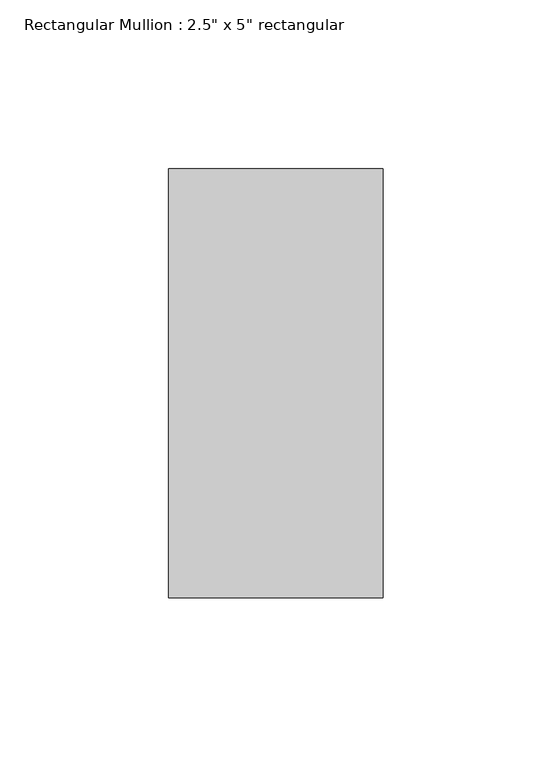
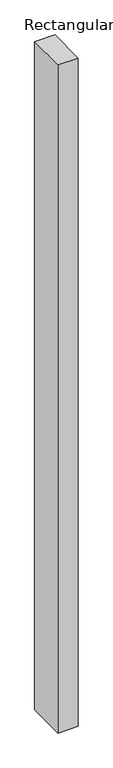
"""IFC4 building model written with IfcOpenShell, lengths in millimetres: member geometry."""

from ifc_helpers import new_model, si_unit, frame, origin, place, context, project, spatial, polyline, outline, extrude, source, transform, mapped, element, save


def member_e6c67f36(model_context):
    return source(origin(), model_context, "Body", "SweptSolid", [
        extrude(outline(polyline([(0.0, 63.5), (0.0, -63.5), (-63.5, -63.5), (-63.5, 63.5), (0.0, 63.5)])), frame((0.0, 0.0, -2224.6166667), z_axis=(0.0, 0.0, 1.0), x_axis=(1.0, 0.0, 0.0)), (0.0, 0.0, 1.0), 2224.6166667),
    ])


if __name__ == "__main__":
    model = new_model("IFC4")
    model_context = context("Model", 3, world=origin())
    ifc_project = project(units=[si_unit("LENGTHUNIT", "METRE", prefix="MILLI")], contexts=[model_context])
    site = spatial("IfcSite", under=ifc_project)
    building = spatial("IfcBuilding", under=site)
    placement = place(None, origin())
    member_shape = member_e6c67f36(model_context)
    element("IfcMember", 1, ObjectType="Rectangular Mullion : 2.5\" x 5\" rectangular", at=placement, inside=building, context=model_context, shape_type="MappedRepresentation", body=[
        mapped(member_shape, transform((0.0, 0.0, 0.0), x_axis=(1.0, 0.0, 0.0), y_axis=(0.0, 1.0, 0.0), z_axis=(0.0, 0.0, 1.0))),
    ])
    save(model, "model.ifc")

# Revit data of these elements
# Type "Rectangular Mullion : 2.5\" x 5\" rectangular"
#   built-in parameter 1007304 = 0.416667 (stored number, unit not read)
#   built-in parameter 1007301 = 0.104167 (stored number, unit not read)
#   built-in parameter 1007300 = 0.104167 (stored number, unit not read)
# Element 1 (IfcMember, "Rectangular Mullion : 2.5\" x 5\" rectangular")
#   Materials on its faces: "Aluminum"
# Materials
#   "Aluminum": class "Metal", colour RGB 247 247 247, transparency 0, Description = "Aluminum 6061", Cost = 0
